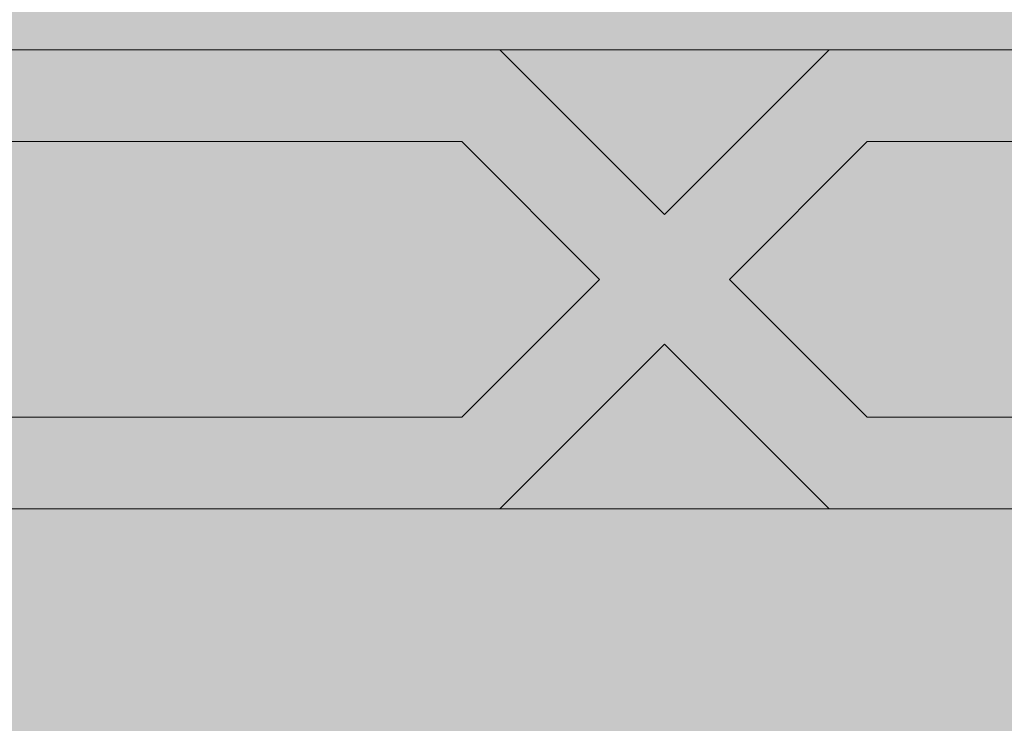
# Model space of a CAD drawing. Units: inches. Extents: x 844 to 2234, y 346 to 1084.
# Tile 81 of 93: x 1999.197 to 2001.933, y 710.971 to 712.926. Entities that reach past the tile are written whole.
import ezdxf

# ---------------------------------------------------------------- set-up
doc = ezdxf.new("R2010")
doc.units = ezdxf.units.IN
doc.header["$MEASUREMENT"] = 0
for name, color, linetype, lineweight in [('A-ANNO-DIMS', 2, 'Continuous', 18), ('furniture', 8, 'Continuous', 18), ('RA-AP-01$0$INT', 35, 'Continuous', 5)]:
    doc.layers.add(name, color=color, linetype=linetype, lineweight=lineweight)
doc.layers.add('RA-AP-01$0$FURN', color=3, linetype='Continuous')
doc.styles.get("Standard").update_dxf_attribs({"font": 'arial.ttf'})
doc.dimstyles.get("Standard").update_dxf_attribs({"dimtxt": 6, "dimasz": 3, "dimexe": 0.18, "dimexo": 0.0625, "dimgap": 0.09, "dimtad": 0, "dimtih": 1, "dimtoh": 1, "dimdec": 1, "dimzin": 0, "dimdsep": 46, "dimlunit": 3, "dimtxsty": 'Standard', "dimblk": 'ARCHTICK', "dimcen": 0.09, "dimadec": 0, "dimazin": 0, "dimtfac": 1, "dimtdec": 1, "dimtofl": 0, "dimtmove": 0, "dimatfit": 3, "dimfxl": 1, "dimtolj": 1, "dimtzin": 0, "dimarcsym": 0})

# ---------------------------------------------------------------- blocks, each defined once
blk = doc.blocks.new('A$C18D01794')
at = {"layer": 'RA-AP-01$0$INT'}
h = blk.add_hatch(color=256, dxfattribs=at)
h.paths.add_polyline_path([(4.355206456958071, -6.156712009588037), (4.355206456958071, -8.056712009588038), (5.455206456958072, -8.056712009588038), (5.455206456958072, -6.156712009588037)])
h.paths.add_polyline_path([(4.405206456958072, -8.006712009588039), (4.405206456958072, -6.206712009588038), (5.405206456958072, -6.206712009588038), (5.405206456958072, -8.006712009588039)], flags=16)
h = blk.add_hatch(color=256, dxfattribs=at)
h.paths.add_polyline_path([(4.505206456958071, -7.585498806127123), (4.46934859260189, -7.549640941759413), (4.505206456958071, -7.513783077414768), (4.505206456958071, -7.381963272220687), (4.469348592616735, -7.346105407867824), (4.505206456958071, -7.310247543514964), (4.505206456958071, -7.178427738324996), (4.469348592586679, -7.142569873965138), (4.505206456952245, -7.106712009588038), (4.476922185709333, -7.106712009588038), (4.455206456960671, -7.128427738343681), (4.433490728198047, -7.106712009588038), (4.405206456946033, -7.106712009588036), (4.441064321339216, -7.142569873969684), (4.40520645695807, -7.178427738362358), (4.405206456958072, -7.310247543472698), (4.441064321364728, -7.346105407867826), (4.40520645695807, -7.381963272262947), (4.40520645695807, -7.513783077378263), (4.441064321354429, -7.549640941786153), (4.405206456958072, -7.585498806170974), (4.405206456958072, -7.717318611286652), (4.441064321333084, -7.753176475673194), (4.405206456958072, -7.789034340036673), (4.405206456958072, -8.006712009588039), (4.644348592588106, -8.006712009588039), (4.680206456964639, -7.970854145211967), (4.716064321341165, -8.006712009588039), (4.869348592586113, -8.006712009588039), (4.905206456964143, -7.970854145210465), (4.941064321342174, -8.006712009588039), (5.094348592587118, -8.006712009588037), (5.130206456963649, -7.970854145211967), (5.166064321340178, -8.006712009588039), (5.405206456958072, -8.006712009588039), (5.405206456958072, -7.789034340024526), (5.369348592595202, -7.753176475673196), (5.40520645695807, -7.717318611298797), (5.40520645695807, -7.585498806158829), (5.369348592573859, -7.549640941786151), (5.40520645695807, -7.51378307739041), (5.40520645695807, -7.381963272250803), (5.36934859256356, -7.346105407867824), (5.405206456958072, -7.310247543484846), (5.405206456958072, -7.178427738350217), (5.369348592589068, -7.142569873969682), (5.405206456982249, -7.106712009588038), (5.376922185730244, -7.106712009588038), (5.355206456967613, -7.128427738343679), (5.333490728218955, -7.10671200958804), (5.305206456976043, -7.106712009588042), (5.341064321341609, -7.142569873965136), (5.305206456958072, -7.178427738337141), (5.305206456958072, -7.310247543502816), (5.34106432131155, -7.346105407867824), (5.305206456958072, -7.381963272232832), (5.30520645695807, -7.513783077402624), (5.341064321326395, -7.549640941759413), (5.305206456958072, -7.585498806139263), (5.305206456958072, -7.717318611299605), (5.341064321347738, -7.753176475677737), (5.305206456958072, -7.78903434007894), (5.30520645695807, -7.906712009588039), (5.166064321336834, -7.906712009588039), (5.130206456963647, -7.942569873961684), (5.094348592590464, -7.906712009588039), (4.941064321338827, -7.906712009588041), (4.905206456964145, -7.942569873963183), (4.869348592589459, -7.906712009588039), (4.716064321337822, -7.906712009588041), (4.680206456964641, -7.942569873961684), (4.644348592591453, -7.906712009588039), (4.505206456958071, -7.906712009588039), (4.505206456958071, -7.789034340066795), (4.469348592580545, -7.753176475677738), (4.505206456958071, -7.717318611311748)])
h.paths.add_polyline_path([(4.485206456974132, -7.709034340046354), (4.45520645695909, -7.739034340051736), (4.425206456974128, -7.709034340057131), (4.425206456993394, -7.593783077384998), (4.45520645699153, -7.563783077396511), (4.485206456993396, -7.593783077408017)], flags=16)
h.paths.add_polyline_path([(4.455206456954537, -7.767318611299197), (4.485206456958242, -7.797318611312542), (4.48520645695951, -7.912569873958716), (4.45520645695415, -7.942569873954422), (4.425206456957888, -7.912569873967813), (4.425206456957888, -7.797318611286197)], flags=16)
h.paths.add_polyline_path([(4.455206456964794, -7.535498806149051), (4.42520645696469, -7.5054988061393), (4.425206456983954, -7.390247543486406), (4.455206456990734, -7.360247543489279), (4.485206456983953, -7.39024754349214), (4.485206456964687, -7.505498806158811)], flags=16)
h.paths.add_polyline_path([(4.499348592588947, -7.926712009585049), (4.636064321340932, -7.926712009585049), (4.666064321342317, -7.956712009586821), (4.636064321343707, -7.986712009585048), (4.499348592575121, -7.986712009585048), (4.469348592591685, -7.956712009591957)], flags=16)
h.paths.add_polyline_path([(4.425206456957888, -7.940854145195974), (4.471064321332215, -7.986712009585049), (4.425206456957888, -7.986712009585049)], flags=16)
h.paths.add_polyline_path([(4.455206456990734, -7.331963272246367), (4.425206456989053, -7.301963272254337), (4.425206456969784, -7.186712009596224), (4.455206456965226, -7.156712009591144), (4.485206456969787, -7.186712009586051), (4.485206456989053, -7.301963272238404)], flags=16)
h.paths.add_polyline_path([(4.72434859258714, -7.926712009586255), (4.861064321340141, -7.926712009586248), (4.891064321340324, -7.956712009586823), (4.861064321340513, -7.986712009586252), (4.724348592586768, -7.986712009586252), (4.694348592586956, -7.956712009586821)], flags=16)
h.paths.add_polyline_path([(4.919348592587961, -7.956712009586821), (4.949348592588145, -7.92671200958625), (5.08606432134115, -7.926712009586253), (5.116064321341327, -7.956712009586823), (5.086064321341519, -7.986712009586252), (4.949348592587774, -7.986712009586252)], flags=16)
h.paths.add_polyline_path([(5.144348592585967, -7.956712009586823), (5.174348592587358, -7.926712009585049), (5.311064321339338, -7.926712009585049), (5.3410643213366, -7.956712009591957), (5.311064321353163, -7.986712009585048), (5.174348592584576, -7.986712009585048)], flags=16)
h.paths.add_polyline_path([(5.32520645693489, -7.593783077408021), (5.355206456936755, -7.563783077396511), (5.385206456934894, -7.593783077384998), (5.38520645695416, -7.709034340057128), (5.355206456969194, -7.739034340051736), (5.325206456954153, -7.709034340046352)], flags=16)
h.paths.add_polyline_path([(5.325206456970042, -7.797318611312542), (5.355206456973747, -7.767318611299197), (5.385206456970398, -7.7973186112862), (5.385206456970398, -7.912569873967816), (5.355206456974136, -7.942569873954422), (5.325206456968778, -7.912569873958716)], flags=16)
h.paths.add_polyline_path([(5.325206456963599, -7.505498806158811), (5.325206456944333, -7.39024754349214), (5.355206456937552, -7.360247543489279), (5.385206456944332, -7.39024754348641), (5.385206456963596, -7.505498806139303), (5.355206456963492, -7.53549880614905)], flags=16)
h.paths.add_polyline_path([(5.32520645693923, -7.301963272238403), (5.3252064569585, -7.186712009586051), (5.355206456963062, -7.156712009591142), (5.3852064569585, -7.186712009596224), (5.385206456939234, -7.301963272254338), (5.355206456937552, -7.331963272246369)], flags=16)
h.paths.add_polyline_path([(5.339348592596071, -7.986712009585048), (5.385206456970398, -7.940854145195972), (5.385206456970396, -7.986712009585048)], flags=16)
h = blk.add_hatch(color=256, dxfattribs=at)
h.paths.add_polyline_path([(4.469348592586677, -7.142569873965136), (4.505206456958073, -7.178427738324996), (4.505206456958071, -7.106712009582215)])
h.paths.add_polyline_path([(4.455206456960671, -7.128427738343681), (4.476922185709333, -7.106712009588038), (4.433490728198045, -7.106712009588038)])
h.paths.add_polyline_path([(4.405206456958073, -7.178427738362358), (4.441064321339218, -7.142569873969684), (4.40520645695807, -7.106712009600073)])
h.paths.add_polyline_path([(4.425206456989053, -7.301963272254335), (4.455206456990736, -7.331963272246371), (4.485206456989055, -7.301963272238399), (4.48520645696979, -7.186712009586054), (4.455206456965227, -7.15671200959114), (4.425206456969784, -7.186712009596224)])
h.paths.add_polyline_path([(4.505206456958073, -7.381963272220689), (4.505206456958071, -7.310247543514961), (4.469348592616738, -7.346105407867826)])
h.paths.add_polyline_path([(4.425206456964688, -7.5054988061393), (4.455206456964794, -7.535498806149051), (4.485206456964689, -7.505498806158811), (4.485206456983951, -7.390247543492138), (4.455206456990736, -7.360247543489277), (4.425206456983956, -7.39024754348641)])
h.paths.add_polyline_path([(4.425206456974126, -7.709034340057128), (4.455206456959092, -7.739034340051736), (4.485206456974132, -7.709034340046356), (4.485206456993396, -7.593783077408017), (4.45520645699153, -7.563783077396511), (4.425206456993394, -7.593783077384999)])
h.paths.add_polyline_path([(4.46934859260189, -7.549640941759415), (4.505206456958071, -7.585498806127123), (4.505206456958073, -7.513783077414766)])
h.paths.add_polyline_path([(4.405206456958073, -7.585498806170972), (4.441064321354427, -7.549640941786151), (4.405206456958072, -7.513783077378263)])
h.paths.add_polyline_path([(4.405206456958072, -7.789034340036673), (4.441064321333084, -7.753176475673194), (4.405206456958072, -7.71731861128665)])
h.paths.add_polyline_path([(4.469348592580547, -7.75317647567774), (4.505206456958071, -7.789034340066795), (4.505206456958071, -7.717318611311744)])
h.paths.add_polyline_path([(4.425206456957888, -7.912569873967814), (4.45520645695415, -7.942569873954422), (4.485206456959507, -7.912569873958718), (4.48520645695824, -7.797318611312542), (4.455206456954537, -7.767318611299197), (4.425206456957888, -7.797318611286202)])
h.paths.add_polyline_path([(4.425206456957888, -7.986712009585049), (4.471064321332215, -7.986712009585049), (4.425206456957888, -7.940854145195972)])
h.paths.add_polyline_path([(4.499348592575121, -7.986712009585048), (4.636064321343707, -7.986712009585049), (4.666064321342317, -7.956712009586823), (4.636064321340932, -7.926712009585049), (4.499348592588945, -7.926712009585049), (4.469348592591685, -7.95671200959196)])
h.paths.add_polyline_path([(4.680206456964641, -7.942569873961684), (4.716064321337824, -7.906712009588039), (4.644348592591454, -7.906712009588039)])
h.paths.add_polyline_path([(4.644348592588108, -8.006712009588039), (4.716064321341167, -8.006712009588039), (4.680206456964637, -7.970854145211964)])
h.paths.add_polyline_path([(4.724348592586768, -7.98671200958625), (4.861064321340514, -7.986712009586252), (4.891064321340324, -7.956712009586819), (4.861064321340141, -7.92671200958625), (4.724348592587134, -7.926712009586255), (4.694348592586957, -7.956712009586821)])
h.paths.add_polyline_path([(4.905206456964143, -7.942569873963183), (4.941064321338827, -7.906712009588039), (4.869348592589457, -7.906712009588037)])
h.paths.add_polyline_path([(4.869348592586113, -8.006712009588039), (4.941064321342172, -8.006712009588037), (4.905206456964145, -7.970854145210463)])
h.paths.add_polyline_path([(4.949348592587774, -7.986712009586252), (5.086064321341521, -7.986712009586252), (5.116064321341329, -7.956712009586823), (5.08606432134115, -7.926712009586253), (4.949348592588145, -7.92671200958625), (4.919348592587961, -7.956712009586819)])
h.paths.add_polyline_path([(5.130206456963645, -7.942569873961684), (5.166064321336834, -7.906712009588039), (5.094348592590464, -7.906712009588039)])
h.paths.add_polyline_path([(5.094348592587119, -8.006712009588039), (5.166064321340178, -8.006712009588039), (5.130206456963651, -7.970854145211967)])
h.paths.add_polyline_path([(5.174348592584578, -7.986712009585048), (5.311064321353163, -7.986712009585048), (5.341064321336602, -7.956712009591958), (5.31106432133934, -7.926712009585049), (5.174348592587352, -7.926712009585049), (5.144348592585969, -7.956712009586823)])
h.paths.add_polyline_path([(5.325206456968778, -7.912569873958718), (5.355206456974136, -7.942569873954422), (5.385206456970396, -7.912569873967814), (5.385206456970396, -7.797318611286199), (5.355206456973747, -7.767318611299197), (5.325206456970044, -7.797318611312544)])
h.paths.add_polyline_path([(5.339348592596073, -7.986712009585048), (5.385206456970396, -7.986712009585049), (5.385206456970398, -7.94085414519597)])
h.paths.add_polyline_path([(5.325206456954155, -7.709034340046354), (5.355206456969194, -7.739034340051734), (5.38520645695416, -7.709034340057128), (5.385206456934896, -7.593783077384999), (5.355206456936758, -7.563783077396513), (5.325206456934888, -7.593783077408019)])
h.paths.add_polyline_path([(5.305206456958072, -7.789034340078938), (5.341064321347739, -7.753176475677738), (5.305206456958072, -7.717318611299605)])
h.paths.add_polyline_path([(5.369348592595204, -7.753176475673194), (5.40520645695807, -7.789034340024526), (5.405206456958072, -7.717318611298798)])
h.paths.add_polyline_path([(5.405206456958072, -7.585498806158831), (5.405206456958072, -7.513783077390407), (5.369348592573857, -7.549640941786151)])
h.paths.add_polyline_path([(5.305206456958072, -7.585498806139266), (5.341064321326393, -7.549640941759413), (5.305206456958072, -7.513783077402626)])
h.paths.add_polyline_path([(5.325206456963599, -7.50549880615881), (5.355206456963494, -7.535498806149055), (5.385206456963598, -7.505498806139302), (5.385206456944334, -7.390247543486411), (5.355206456937552, -7.360247543489279), (5.325206456944333, -7.39024754349214)])
h.paths.add_polyline_path([(5.305206456958072, -7.38196327223283), (5.341064321311551, -7.346105407867824), (5.305206456958072, -7.31024754350282)])
h.paths.add_polyline_path([(5.325206456939231, -7.301963272238404), (5.355206456937552, -7.331963272246369), (5.385206456939235, -7.301963272254335), (5.385206456958502, -7.186712009596224), (5.355206456963061, -7.156712009591142), (5.3252064569585, -7.186712009586051)])
h.paths.add_polyline_path([(5.404581768715993, -7.381338584008926, -0.001217816984214), (5.405206456958072, -7.381112009582329), (5.405206456958072, -7.310247543484846), (5.369348592563558, -7.346105407867826)])
h.paths.add_polyline_path([(5.36934859258907, -7.142569873969684), (5.40520645695807, -7.178427738350215), (5.405206456958072, -7.106712009612218)])
h.paths.add_polyline_path([(5.355206456967613, -7.128427738343683), (5.376922185730239, -7.106712009588038), (5.333490728218953, -7.10671200958804)])
h.paths.add_polyline_path([(5.30520645695807, -7.178427738337139), (5.341064321341609, -7.142569873965134), (5.305206456958074, -7.10671200957007)])
blk.add_hatch(color=256, dxfattribs=at).paths.add_polyline_path([(4.505206456958071, -7.906712009588039), (5.305206456958072, -7.906712009588039), (5.305206456958072, -7.106712009588038), (5.255206456951893, -7.106712009588036), (5.25520645694868, -7.856712009570104), (4.555206456959269, -7.856712009588616), (4.555206456956052, -7.106712009588038), (4.505206456958073, -7.106712009588038)])
for p, q in [((5.267206456961765, -7.906712009586254), (4.543206456966523, -7.906712009586254)), ((5.2672064569642, -7.906712009586255), (4.54320645696085, -7.906712009586255)), ((5.094348592588679, -7.906712009586254), (5.130206456963647, -7.942569873961684)), ((5.166064321338619, -7.906712009586254), (5.130206456963647, -7.942569873961684)), ((4.949348592588145, -7.92671200958625), (5.08606432134115, -7.926712009586253)), ((5.08606432134115, -7.926712009586253), (5.116064321341329, -7.956712009586823)), ((5.174348592587354, -7.926712009585049), (5.144348592585969, -7.956712009586823)), ((5.174348592587354, -7.926712009585049), (5.31106432133934, -7.926712009585049)), ((5.086064321341518, -7.986712009586252), (5.116064321341329, -7.956712009586823)), ((5.174348592584578, -7.986712009585049), (5.144348592585969, -7.956712009586823)), ((5.094348592588905, -8.006712009586252), (5.130206456963649, -7.970854145211966)), ((5.166064321338393, -8.006712009586252), (5.130206456963649, -7.970854145211966)), ((4.949348592587774, -7.986712009586252), (5.086064321341518, -7.986712009586252)), ((5.174348592584578, -7.986712009585049), (5.311064321353163, -7.986712009585048))]:
    blk.add_line(p, q, dxfattribs=at)
for points in [[(5.405206456958072, -8.006712009588039), (4.405206456958072, -8.006712009588039), (4.405206456958072, -7.106712009588038)], [(5.305206456958072, -7.106712009588038), (5.305206456958072, -7.906712009588039), (4.505206456958071, -7.906712009588039), (4.505206456958071, -7.106712009588038)]]:
    blk.add_lwpolyline(points, dxfattribs=at)
blk = doc.blocks.new('A$C5D2F253E')
at = {"layer": 'RA-AP-01$0$FURN', "xscale": -0.7999999999883585, "yscale": 0.7999999999883585, "zscale": 0.8, "rotation": 90}
blk.add_blockref('A$C18D01794', (-5.687757199772477, 4.75791982714071), dxfattribs=at)
blk = doc.blocks.new('_ArchTick')
at = {"color": 0, "linetype": 'ByBlock', "const_width": 0.15}
blk.add_lwpolyline([(-0.5, -0.5), (0.5, 0.5)], dxfattribs=at)
blk = doc.blocks.new('*D121')
at = {"layer": 'A-ANNO-DIMS', "color": 0, "lineweight": -2, "transparency": 16777216}
for p, q in [((2030.271987351997, 734.262611118704), (2040.245275089302, 734.262611118704)), ((2040.065275089302, 734.262611118704), (2040.065275089302, 704.6043509484256)), ((2040.065275089302, 668.557359536674), (2040.065275089302, 698.2156197069523)), ((2030.271987351997, 668.557359536674), (2040.245275089302, 668.557359536674))]:
    blk.add_line(p, q, dxfattribs=at)
at = {"layer": 'Defpoints', "color": 0, "transparency": 16777216}
for p in [(2030.209487351997, 734.262611118704), (2040.065275089302, 734.262611118704), (2030.209487351997, 668.557359536674)]:
    blk.add_point(p, dxfattribs=at)
at = {"layer": 'A-ANNO-DIMS', "color": 0, "lineweight": -2, "transparency": 16777216, "xscale": 3, "yscale": 3, "zscale": 3}
for p, rotation in [((2040.065275089302, 734.262611118704), 90), ((2040.065275089302, 668.557359536674), 270)]:
    blk.add_blockref('_ArchTick', p, dxfattribs=dict(at, rotation=rotation))
at = {"layer": 'A-ANNO-DIMS', "color": 0, "transparency": 16777216, "insert": (2040.065275089302, 701.4099853276883), "char_height": 6, "attachment_point": 5}
blk.add_mtext('\\A1;LOUNGE SET 5\'-5 1/2" TYP.', dxfattribs=at)

msp = doc.modelspace()

# ---------------------------------------------------------------- block references
at = {"layer": 'furniture', "xscale": -15.94108302203742, "yscale": 15.94108302203742, "zscale": 15.94108302203742, "rotation": 270}
msp.add_blockref('A$C5D2F253E', (1990.567271852805, 701.4028671565849), dxfattribs=at)

# ---------------------------------------------------------------- dimensions: what is measured, and where the dimension line sits
at = {"layer": 'A-ANNO-DIMS'}
dim = msp.add_linear_dim(base=(2040.065275089302, 734.262611118704), p1=(2030.209487351996, 668.5573595366737), p2=(2030.209487351996, 734.2626111187037), angle=90, text='LOUNGE SET <> TYP.', dimstyle='Standard', override={"dimdec": 1, "dimlfac": 1, "dimrnd": 0, "dimzin": 1, "dimdsep": 46, "dimlunit": 4, "dimfrac": 2}, dxfattribs=at)
dim.commit()
dim.dimension.update_dxf_attribs({"geometry": '*D121', "text_midpoint": (2040.065275089302, 701.4099853276883)})

doc.saveas('drawing.dxf')
